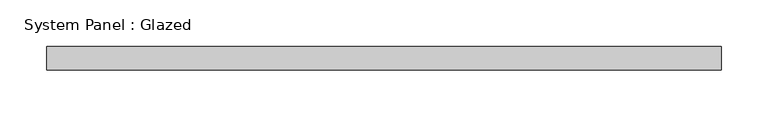
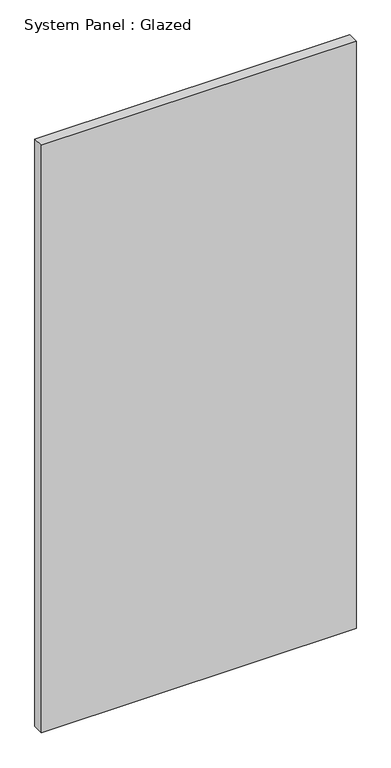
"""IFC4 building model written with IfcOpenShell, lengths in millimetres: plate geometry, System Panel : Glazed."""

from ifc_helpers import new_model, si_unit, origin, origin_with_axes, place, context, project, spatial, polyline, outline, extrude, source, transform, mapped, element, save


def system_panel_glazed_07b088f8(model_context):
    return source(origin(), model_context, "Body", "SweptSolid", [
        extrude(outline(polyline([(362.0017238, 19.05), (-362.0017238, 19.05), (-362.0017238, 44.45), (362.0017238, 44.45), (362.0017238, 19.05)])), origin_with_axes(), (0.0, 0.0, 1.0), 1428.75),
    ])


if __name__ == "__main__":
    model = new_model("IFC4")
    model_context = context("Model", 3, world=origin())
    ifc_project = project(units=[si_unit("LENGTHUNIT", "METRE", prefix="MILLI")], contexts=[model_context])
    site = spatial("IfcSite", under=ifc_project)
    building = spatial("IfcBuilding", under=site)
    placement = place(None, origin())
    system_panel_glazed_shape = system_panel_glazed_07b088f8(model_context)
    element("IfcPlate", 1, ObjectType="System Panel : Glazed", at=placement, inside=building, context=model_context, shape_type="MappedRepresentation", body=[
        mapped(system_panel_glazed_shape, transform((0.0, 0.0, 0.0), x_axis=(1.0, 0.0, 0.0), y_axis=(0.0, 1.0, 0.0), z_axis=(0.0, 0.0, 1.0))),
    ])
    save(model, "model.ifc")

# Revit data of these elements
# Type "System Panel : Glazed"
#   Construction Type Id = "GSP4R"
#   Analytic Construction = "1/8 in Pilkington single glazing"
#   Visual Light Transmittance = 0.9
#   Solar Heat Gain Coefficient = 0.86
#   Heat Transfer Coefficient (U) = 1.18115 BTU/(h·ft²·°F)
#   Define Thermal Properties by = 1
# Element 1 (IfcPlate, "System Panel : Glazed")
#   Materials on its faces: "Glass"
# Materials
#   "Glass": class "Glass", colour RGB 0 128 192, transparency 0.75, Description = "Soda Lime Glass", Cost = 0
